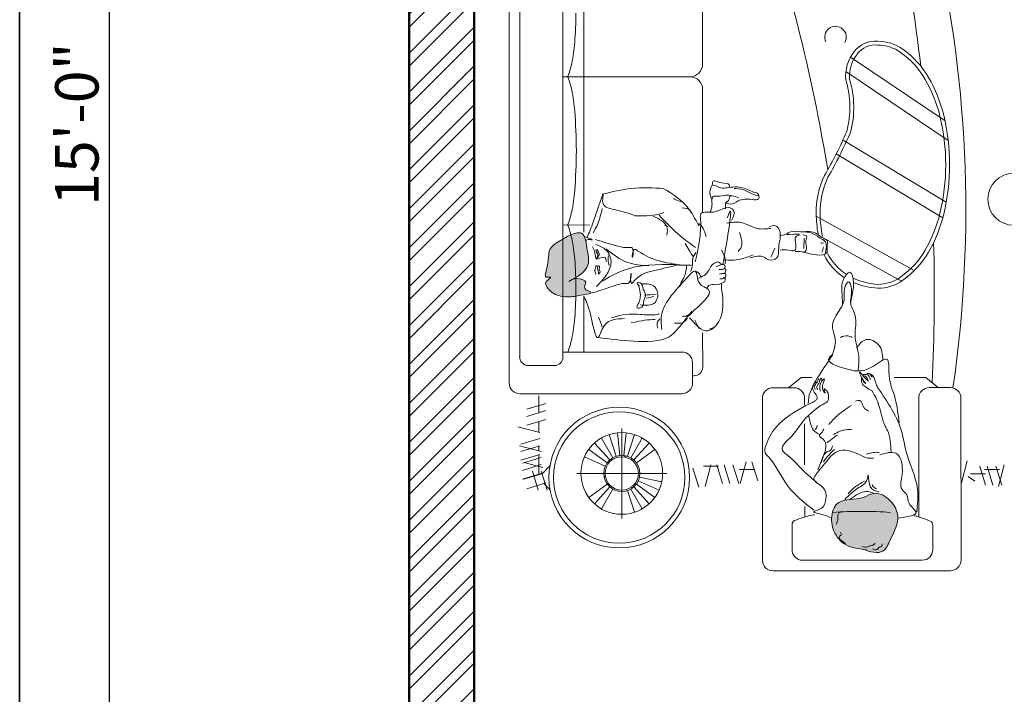
# Model space of a CAD drawing. Units: millimetres. Extents: x 20768 to 23556, y 50760 to 52704.
# Tile 16 of 36: x 21272 to 21408, y 51912 to 52005. Entities that reach past the tile are written whole.
import ezdxf

# ---------------------------------------------------------------- set-up
doc = ezdxf.new("R2010")
doc.units = ezdxf.units.MM
for name, color, linetype, lineweight in [('A-ANNO-TTLB', 7, 'Continuous', 35), ('A-FURN', 8, 'Continuous', 18), ('A-WALL', 7, 'Continuous', 50), ('A-WALL-PATT', 8, 'Continuous', 13), ('S-ANNO-DIMS', 2, 'Continuous', 18)]:
    doc.layers.add(name, color=color, linetype=linetype, lineweight=lineweight)
doc.styles.get("Standard").update_dxf_attribs({"font": 'arial.ttf'})
doc.dimstyles.new('ISO-25', dxfattribs={"dimtxt": 6, "dimasz": 2.5, "dimexe": 1.25, "dimexo": 0.625, "dimtad": 1, "dimdec": 0, "dimlunit": 3, "dimtxsty": 'Standard', "dimcen": 2.5, "dimadec": 0, "dimazin": 0, "dimtfac": 1, "dimtdec": 0, "dimtmove": 0, "dimatfit": 3, "dimfxl": 1, "dimarcsym": 0})

# ---------------------------------------------------------------- blocks, each defined once
blk = doc.blocks.new('A$C32DD204E')
at = {"ltscale": 3}
h = blk.add_hatch(color=256, dxfattribs=at)
edge = h.paths.add_edge_path()
edge.add_spline(control_points=[(248.5, 1171), (279.6, 1188.5), (331.5, 1220.4), (312.1, 1296.2), (303.9, 1374.7), (243.4, 1354.4), (209.2, 1331.9), (147.9, 1299.6), (163.4, 1244.6), (138.6, 1178), (180.2, 1188.1), (136, 1164), (157.4, 1133.7), (185.5, 1110.9), (241.5, 1099.6), (276.6, 1109.9), (350.3, 1120.6), (292.2, 1133.5), (320.4, 1170.6), (274.8, 1182.2), (255.2, 1174.5), (248.5, 1171)], knot_values=[6.92976, 6.92976, 6.92976, 6.92976, 88.633957, 150.80248, 204.81141, 248.139794, 279.389018, 321.893636, 408.375761, 431.643524, 447.144857, 469.07466, 497.305108, 522.125936, 570.063074, 628.708388, 656.922664, 684.873946, 704.64736, 740.083308, 760.727208, 760.727208, 760.727208, 760.727208], degree=3, periodic=0)
h = blk.add_hatch(color=256, dxfattribs=at)
edge = h.paths.add_edge_path()
edge.add_spline(control_points=[(1426.4, 86.6), (1397.7, 90.1), (1345.7, 99.1), (1298.9, 165.8), (1296.3, 225.7), (1328.2, 297.6), (1410.2, 279.3), (1477.3, 324.4), (1540.8, 288.1), (1580.5, 210.8), (1543, 141.8), (1506.8, 60.6), (1456.5, 76.7), (1426.4, 86.6)], knot_values=[11.171972, 11.171972, 11.171972, 11.171972, 83.935274, 146.390702, 207.043537, 236.474222, 338.687878, 374.142978, 438.985032, 497.846364, 587.349285, 634.808067, 704.959464, 704.959464, 704.959464, 704.959464], degree=3, periodic=0)
for p, q in [((0, 755.3, -685.7), (0.2, 2629.6, -685.7)), ((779.4, 2042.5, -685.7), (779.6, 2565.6, -685.7)), ((42.1, 861.2, -685.7), (42.7, 2524.3, -685.7)), ((216, 1393.9, -685.7), (216.2, 2524.2, -685.7)), ((301, 1394, -685.7), (301.2, 2504.1, -685.7)), ((1375.8, 2071.1, -685.7), (1756.4, 1813.8, -685.7)), ((216, 1991.7, -685.7), (595.7, 1991.5, -685.7)), ((595.7, 1991.5, -685.7), (728.3, 1991.5, -685.7)), ((1356.9, 2013.1, -685.7), (1769.1, 1734.5, -685.7)), ((779.4, 1940.4, -685.7), (779.4, 1445.2, -685.7)), ((1345.3, 1735.8, -685.7), (1761.4, 1485.6, -685.7)), ((1318.2, 1681.4, -685.7), (1747.5, 1423.2, -685.7)), ((1237.5, 1428.9, -685.7), (1632.1, 1210.6, -685.7)), ((216, 1394.2, -685.7), (216.2, 861.4, -685.7)), ((216, 1393.9, -685.7), (323, 1394, -685.7)), ((301, 1394.2, -685.7), (301, 1364.8, -685.7)), ((1245.7, 1353.6, -685.7), (1581.4, 1167.9, -685.7)), ((1188.7, 1340.5), (1187.5, 1298.8)), ((301.1, 1106.9, -685.7), (301.2, 881.5, -685.7)), ((370.5, 964.2), (368.9, 965.7)), ((779.5, 959.1, -685.7), (779.6, 820, -685.7)), ((216.2, 881.5, -685.7), (696.3, 881.7, -685.7)), ((738.8, 782.8, -685.7), (738.8, 839.2, -685.7)), ((76.8, 827.3, -685.7), (182.2, 827.3, -685.7)), ((739.1, 787, -685.7), (739.1, 756.3, -685.7)), ((739.1, 785.9, -685.7), (745.6, 785.9, -685.7)), ((1125.7, 738.2, -685.7), (1176, 779.7, -685.7)), ((1220.3, 779.7, -685.7), (1176, 779.7, -685.7)), ((1678.7, 779.9, -685.7), (1551.9, 779.9, -685.7)), ((1729.9, 737.7, -685.7), (1678.7, 779.9, -685.7)), ((1148, 738.2, -685.7), (1062.9, 738.1, -685.7)), ((1778.1, 738.4, -685.7), (1693.1, 738.4, -685.7)), ((42.8, 713.5, -685.7), (696.6, 713.7, -685.7)), ((147, 675, -685.7), (70.5, 651.5, -685.7)), ((1020.4, 695.6, -685.7), (1020.7, 42.5, -685.7)), ((1190.5, 669.7, -685.7), (1190.5, 695.7, -685.7)), ((1650.7, 217.2, -685.7), (1650.6, 695.8, -685.7)), ((1820.9, 42.8, -685.7), (1820.7, 695.9, -685.7)), ((147, 645.6, -685.7), (70.5, 622.1, -685.7)), ((147, 610.3, -685.7), (70.5, 586.8, -685.7)), ((123.5, 557.3, -685.7), (35.3, 580.9, -685.7)), ((446, 465, -685.7), (436.4, 556.4, -685.7)), ((453.6, 392.6, -685.7), (453.6, 574.3, -685.7)), ((461.2, 465, -685.7), (470.8, 556.4, -685.7)), ((1190.6, 427.1, -685.7), (1190.6, 592.2, -685.7)), ((123.5, 533.8, -685.7), (47, 510.3, -685.7)), ((417.2, 455.6, -685.7), (371.3, 535.2, -685.7)), ((431.1, 461.8, -685.7), (402.7, 549.2, -685.7)), ((476.1, 461.8, -685.7), (504.5, 549.2, -685.7)), ((490, 455.6, -685.7), (536, 535.2, -685.7)), ((129.3, 480.9, -685.7), (41.1, 504.4, -685.7)), ((123.5, 504.4, -685.7), (47, 480.9, -685.7)), ((394.8, 435.4, -685.7), (320.4, 489.4, -685.7)), ((404.9, 446.7, -685.7), (343.4, 515, -685.7)), ((502.3, 446.7, -685.7), (563.8, 515, -685.7)), ((512.5, 435.4, -685.7), (586.9, 489.4, -685.7)), ((123.5, 469.1, -685.7), (47, 445.6, -685.7)), ((129.3, 457.3, -685.7), (52.9, 433.8, -685.7)), ((387.1, 422.2, -685.7), (303.2, 459.6, -685.7)), ((469.9, 463.5, -685.7), (465.2, 458.8, -685.7)), ((954.3, 439.6, -685.7), (930.7, 351.4, -685.7)), ((977.8, 439.6, -685.7), (1001.3, 363.1, -685.7)), ((1822.4, 354.9, -685.7), (1846, 443.1, -685.7)), ((129.3, 427.9, -685.7), (52.9, 404.4, -685.7)), ((135.2, 416.2, -685.7), (60.4, 436.1, -685.7)), ((117, 325.5, -685.7), (93.5, 401.9, -685.7)), ((152.3, 325.5, -685.7), (128.8, 401.9, -685.7)), ((163.9, 422.7, -685.7), (132.1, 390.9, -685.7)), ((764.1, 337.3, -685.7), (740.6, 413.7, -685.7)), ((783.1, 421.6), (843.8, 421.6)), ((813.1, 427.8, -685.7), (789.5, 339.6, -685.7)), ((836.6, 427.8, -685.7), (860.1, 351.4, -685.7)), ((866, 427.8, -685.7), (889.5, 351.4, -685.7)), ((901.3, 427.8, -685.7), (924.8, 351.4, -685.7)), ((928.1, 408.1), (988.8, 408.1)), ((1896.4, 421.9, -685.7), (1920, 345.5, -685.7)), ((1915.9, 408.1), (1976.6, 408.1)), ((1925.8, 421.9, -685.7), (1949.4, 345.5, -685.7)), ((1961.1, 421.9, -685.7), (1984.7, 345.5, -685.7)), ((1995.1, 427.8, -685.7), (1971.6, 339.6, -685.7)), ((129.3, 392.6, -685.7), (52.9, 369.1, -685.7)), ((135.2, 392.6, -685.7), (58.8, 369.1, -685.7)), ((453.6, 392.6, -685.7), (271.9, 392.6, -685.7)), ((387.4, 381, -685.7), (382.7, 376.3, -685.7)), ((453.6, 392.6, -685.7), (453.6, 210.9, -685.7)), ((453.6, 392.6, -685.7), (635.4, 392.6, -685.7)), ((520.1, 363, -685.7), (604.1, 325.6, -685.7)), ((524.8, 377.5, -685.7), (614.7, 358.3, -685.7)), ((1849.9, 380.2, -685.7), (1876.3, 360.8, -685.7)), ((1858.6, 391.3), (1919.3, 391.3)), ((147, 354.5, -685.7), (70.5, 331, -685.7)), ((139.9, 352.3, -685.7), (164.1, 328, -685.7)), ((394.8, 349.8, -685.7), (320.4, 295.8, -685.7)), ((404.9, 338.5, -685.7), (343.4, 270.2, -685.7)), ((417.2, 329.6, -685.7), (371.3, 249.9, -685.7)), ((476.1, 323.4, -685.7), (504.5, 235.9, -685.7)), ((490, 329.6, -685.7), (536, 249.9, -685.7)), ((502.3, 338.5, -685.7), (563.8, 270.2, -685.7)), ((512.5, 349.8, -685.7), (586.9, 295.8, -685.7)), ((1190.7, 217.1, -685.7), (1190.7, 258.6, -685.7)), ((1139.7, 85.1, -685.7), (1139.7, 186.8, -685.7)), ((1707.1, 85.3, -685.7), (1707, 184.5, -685.7)), ((1182.2, 42.6, -685.7), (1664.6, 42.8, -685.7)), ((1063.2, 0, -685.7), (1778.4, 0.3, -685.7))]:
    blk.add_line(p, q)
at = {"elevation": -685.7}
for points in [[(234.8, 1392.4, 0.047423), (251.7, 1447.7, 0.029233), (263.9, 1532.1, 0.017749), (270.5, 1692.8, 0.02107)], [(234.8, 1395.5, -0.047423), (251.7, 1340.2, -0.029233), (263.9, 1255.7, -0.02107), (268.9, 1137.6, -0.02107)], [(236, 1394.2, -0.00246), (234.8, 1391.4)], [(268.9, 1137.6, -0.02107), (264, 1019.4, -0.029233), (251.9, 935, -0.045778), (235.8, 881.5, -0.201615)]]:
    blk.add_lwpolyline(points, format="xyb", dxfattribs=at)
for points in [[(119.4, 705.9), (119.4, 637.1)], [(119.4, 601.8), (119.4, 558.4)], [(119.4, 503.2), (119.4, 483.5)], [(119.4, 467.9), (119.4, 387.8)]]:
    blk.add_lwpolyline(points, dxfattribs=at)
for centre, radius in [((2033.7, 1497.8, -685.7), 104.7), ((443.5, 376, -685.7), 283.5), ((443.5, 376, -685.7), 264.6), ((453.6, 392.6, -685.7), 164.7), ((453.6, 392.6, -685.7), 72.8), ((453.6, 392.6, -685.7), 67.2)]:
    blk.add_circle(centre, radius)
for centre, radius, start, end in [((-3160.4, 1453.5, -685.7), 5000.5, 351.7639, 13.5399), ((-5717.4, 460.8, -685.7), 7095.9, 9.37507, 17.5955), ((-6034.3, 1118.6, -685.7), 7747.5, 6.78419, 11.06631), ((-1135.1, 2248.6, -685.7), 1404, 355.1489, 359.9772), ((1315, 2151.6, -685.7), 43.3, 329.4196, 206.4089), ((-463.5, 2191.6, -685.7), 730, 348.451, 355.1489), ((1474.3, 2030.8, -685.7), 104.3, 83.9251, 143.2199), ((1474.3, 2030.8, -685.7), 88.8, 83.3999, 143.3893), ((1485.3, 1960, -685.7), 159, 54.5394, 90.3034), ((1485.3, 1960, -685.7), 174.6, 54.5394, 90), ((1514.9, 1993.6, -685.7), 159.2, 141.263, 185.4473), ((1514.9, 1993.6, -685.7), 143.6, 141.1552, 184.8436), ((1375.6, 1805.9, -685.7), 348.1, 30.1802, 54.5394), ((1375.6, 1805.9, -685.7), 363.7, 30.1802, 54.5394), ((-47.7, 2106.6, -685.7), 305.7, 337.5906, 348.451), ((728.3, 2042.5, -685.7), 51, 269.9772, 359.9772), ((-47.8, 1877.9, -685.7), 305.7, 21.7999, 22.3637), ((-47.7, 1876.7, -685.7), 305.7, 11.549, 22.4094), ((728.3, 1940.4, -685.7), 51, 0.0228, 90.0228), ((1200.1, 1703.8, -685.7), 566.7, 13.5438, 30.1802), ((993.4, 1867.9, -685.7), 379.5, 345.261, 16.9432), ((993.4, 1867.9, -685.7), 395.1, 345.0883, 16.7074), ((1200.1, 1703.8, -685.7), 551.1, 13.5438, 30.1802), ((-463.5, 1791.7, -685.7), 730, 4.8511, 11.549), ((-1995, 1680, -685.7), 2265.5, 0.3248, 4.3921), ((921.7, 1636.8, -685.7), 837.4, 0, 13.5438), ((921.7, 1636.8, -685.7), 853, 0, 13.5438), ((-174.4, 2435.8, -685.7), 1672.4, 329.7762, 336.5922), ((-174.4, 2435.8, -685.7), 1688, 329.7992, 336.632), ((921.7, 1636.8, -685.7), 837.4, 346.4562, 0), ((921.7, 1636.8, -685.7), 853, 346.4562, 0), ((1584.9, 1445.2, -685.7), 347.6, 154.6827, 181.0708), ((1584.9, 1445.2, -685.7), 332, 154.7964, 181.089), ((1699.8, 1441.1, -685.7), 462.4, 180.2965, 190.3289), ((1699.8, 1441.1, -685.7), 446.9, 180.283, 192.0106), ((1200.1, 1569.7, -685.7), 551.1, 329.8198, 346.4562), ((1200.1, 1569.7, -685.7), 566.7, 329.8198, 346.4562), ((464.9, -539.7), 1961.2, 81.0036, 81.3607), ((631.8, -596.5), 1995.1, 85.9802, 86.2563), ((-6034.3, 1118.6, -685.7), 7747.5, 357.33463, 1.51542), ((1486, 1384.5, -685.7), 244, 207.1509, 235.8302), ((1486, 1384.5, -685.7), 228.4, 207.3492, 235.7987), ((1375.6, 1467.7, -685.7), 348.1, 305.4606, 329.8198), ((1375.6, 1467.7, -685.7), 363.7, 305.4606, 329.8198), ((1509.1, 1466.2, -685.7), 312.4, 247.051, 265.7344), ((1509.1, 1466.2, -685.7), 328, 248.6473, 265.8394), ((1485.3, 1313.6, -685.7), 174.6, 270, 305.4606), ((1485.3, 1313.6, -685.7), 159, 270.2019, 305.4606), ((696.3, 839.1, -685.7), 42.5, 0.0228, 90.0228), ((77.2, 862.5, -685.7), 35.2, 177.8872, 269.238), ((182.2, 861.4, -685.7), 34, 270.0228, 0.0228), ((745.5, 820, -685.7), 34, 270.0228, 0.0228), ((42.9, 756.4, -685.7), 42.9, 178.4457, 269.7882), ((696.5, 756.3, -685.7), 42.5, 270.0228, 0.0228), ((1063, 695.6, -685.7), 42.5, 90.0228, 180.0228), ((1148, 695.6, -685.7), 42.5, 0.0228, 90.0228), ((1693.1, 695.9, -685.7), 42.5, 90.0228, 180.0228), ((1778.1, 695.9, -685.7), 42.5, 0.0228, 90.0228), ((1421.2, -1279.2, -685.7), 1518.9, 90.0228, 94.419), ((1421.2, -1279.2, -685.7), 1518.9, 85.6266, 90.0228), ((1156.7, 186.8, -685.7), 17, 113.7374, 180.0228), ((1280.5, -94.8, -685.7), 324.6, 100.5374, 113.7374), ((1364.6, -547, -685.7), 784.5, 99.8363, 100.5374), ((1560.9, -94.7, -685.7), 324.6, 65.1817, 77.2735), ((1690, 184.5, -685.7), 17, 0.0228, 65.1817), ((1182.2, 85.1, -685.7), 42.5, 180.0228, 270.0228), ((1664.6, 85.3, -685.7), 42.5, 270.0228, 0.0228), ((1063.2, 42.5, -685.7), 42.5, 180.0228, 270.0228), ((1778.4, 42.8, -685.7), 42.5, 270.0228, 0.0228)]:
    blk.add_arc(centre, radius, start, end)
at = {"ltscale": 3}
for centre, radius, start, end in [((1357, 906.6), 40.6, 79.5148, 123.0894), ((1352, 880), 67.7, 63.6392, 79.5148)]:
    blk.add_arc(centre, radius, start, end, dxfattribs=at)
for points, knots in [([(815.6, 1499.7), (813.2, 1505.1), (807.5, 1517.9), (809.7, 1535.9), (818.3, 1563.8), (849.5, 1539.3), (888.8, 1546.3), (939.9, 1551.3), (976, 1527), (1006.1, 1522.5), (1011, 1491), (964.4, 1500), (925.8, 1499.2), (898.4, 1471.9), (869.3, 1485.1), (891, 1492.1), (886, 1512.2), (894.6, 1511.6), (895.6, 1511.5)], [0, 0, 0, 0, 15.214729, 36.055512, 48.857472, 79.738512, 103.122769, 157.685733, 206.194273, 214.411126, 234.296897, 257.825245, 307.464974, 341.56748, 352.042995, 362.192251, 380.803332, 383.401633, 383.401633, 383.401633, 383.401633]), ([(817.1, 1553), (818.2, 1556.2), (819.7, 1561), (820, 1579.5), (854.5, 1556.5), (888.8, 1565.3), (887.1, 1549.5), (886.7, 1545.6)], [0, 0, 0, 0, 9.109215, 13.285838, 44.707752, 72.752889, 81.852859, 81.852859, 81.852859, 81.852859]), ([(314.5, 1345.5), (321.9, 1362.7), (341.1, 1407.4), (387.3, 1556.5), (369.3, 1464.2), (445.2, 1454.4), (487.7, 1439.1), (511.9, 1430.4)], [0, 0, 0, 0, 60.518576, 156.742964, 182.299185, 237.275016, 309.902587, 309.902587, 309.902587, 309.902587]), ([(374.5, 1517.7), (413.9, 1527.5), (495.5, 1547.9), (579.6, 1543.7), (622.9, 1541.5)], [0, 0, 0, 0, 106.409885, 220.025525, 220.025525, 220.025525, 220.025525]), ([(623, 1540.2), (656.5, 1519.3), (716.8, 1481.5), (749.4, 1418.6), (764, 1390.6)], [0, 0, 0, 0, 101.553402, 183.196527, 183.196527, 183.196527, 183.196527]), ([(809.7, 1446.3), (813.1, 1455.2), (819.4, 1471.8), (815.4, 1492.1), (820.4, 1513), (846.6, 1507.3), (878.7, 1519.8), (907.7, 1510), (925.2, 1504.1)], [0, 0, 0, 0, 24.284632, 45.084884, 56.190964, 71.83444, 101.967681, 148.338712, 148.338712, 148.338712, 148.338712]), ([(906, 1541.1), (918.1, 1540.7), (943.5, 1539.6), (973.1, 1520.3), (994.7, 1514.1), (1003.7, 1511.5)], [0, 0, 0, 0, 31.421868, 65.723795, 90.374568, 90.374568, 90.374568, 90.374568]), ([(662.7, 1500.2), (666.7, 1498), (679.3, 1491.4), (693.1, 1487.5), (702.4, 1484.9)], [0, 0, 0, 0, 12.001288, 37.458402, 37.458402, 37.458402, 37.458402]), ([(895.2, 1411.9), (903.3, 1427.4), (912.7, 1445.6), (880, 1477.1), (837.9, 1433.9), (767.6, 1451.2), (776.7, 1361.9), (762.8, 1301.5), (749.8, 1245.2)], [0, 0, 0, 0, 37.77004, 44.330448, 112.206702, 158.127425, 169.373671, 326.046663, 326.046663, 326.046663, 326.046663]), ([(861.3, 1235.3), (864.2, 1253), (878.2, 1331.2), (903.8, 1491.5), (882.2, 1430.6), (879.3, 1422.5)], [229.252261, 229.252261, 229.252261, 229.252261, 259.312026, 344.867622, 358.082672, 358.082672, 358.082672, 358.082672]), ([(871.9, 1484.8), (871.9, 1477.9), (871.9, 1469.5), (871.9, 1461.1), (871.9, 1459.6)], [0, 0, 0, 0, 18.199941, 22.100035, 22.100035, 22.100035, 22.100035]), ([(338.4, 1362.4), (345, 1374.5), (361.7, 1405.4), (370, 1439.6), (375.1, 1460.4)], [0, 0, 0, 0, 36.019014, 92.081432, 92.081432, 92.081432, 92.081432]), ([(505.6, 1431.2), (538.2, 1430.5), (578.2, 1429.6), (616, 1441.7), (623, 1444)], [0, 0, 0, 0, 84.476355, 104.032988, 104.032988, 104.032988, 104.032988]), ([(580.1, 1429.8), (591.5, 1424.4), (612.6, 1414.6), (640.6, 1388.2), (637, 1365), (635.1, 1353.2)], [0, 0, 0, 0, 33.626167, 62.160116, 91.695701, 91.695701, 91.695701, 91.695701]), ([(603.8, 1433.3), (631.3, 1404.4), (676.7, 1356.7), (730.1, 1318.2), (751.2, 1303)], [0, 0, 0, 0, 104.676597, 172.875133, 172.875133, 172.875133, 172.875133]), ([(696.3, 1463.4), (710.4, 1462.2), (728.4, 1460.6), (732.2, 1445.3), (733, 1442)], [0, 0, 0, 0, 31.408902, 39.899476, 39.899476, 39.899476, 39.899476]), ([(772.8, 1393), (778.4, 1384.1), (787.5, 1369.7), (792.4, 1353.3), (794.2, 1347.1)], [0, 0, 0, 0, 27.640179, 44.620551, 44.620551, 44.620551, 44.620551]), ([(877.4, 1401.3), (897.1, 1404.5), (939.9, 1411.6), (993.7, 1373.5), (1035.6, 1378.1), (1054.5, 1380.1)], [0, 0, 0, 0, 51.063738, 110.501338, 159.193788, 159.193788, 159.193788, 159.193788]), ([(969.9, 1261.1), (990.7, 1266.8), (1019.1, 1274.6), (1048.1, 1247.4), (1089.5, 1258.3), (1081.3, 1314.7), (1101.6, 1357.4), (1073.7, 1397.1), (1055.9, 1389.4), (1046.5, 1385.4)], [0, 0, 0, 0, 51.063966, 69.760857, 98.442485, 136.21289, 196.583877, 217.96974, 241.616381, 241.616381, 241.616381, 241.616381]), ([(240.5, 1166.5), (274.5, 1185.5), (332.2, 1217.8), (312.1, 1296.2), (303.9, 1374.7), (243.4, 1354.4), (209.2, 1331.9), (147.9, 1299.6), (163.4, 1244.6), (138.6, 1178), (180.2, 1188.1), (136, 1164), (157.4, 1133.7), (185.5, 1110.9), (241.5, 1099.6), (276.6, 1109.9), (350.3, 1120.6), (292.2, 1133.5), (320.4, 1170.6), (269.8, 1183.5), (249.6, 1171.8), (240.5, 1166.5)], [0, 0, 0, 0, 88.633957, 150.80248, 204.81141, 248.139794, 279.389018, 321.893636, 408.375761, 431.643524, 447.144857, 469.07466, 497.305108, 522.125936, 570.063074, 628.708388, 656.922664, 684.873946, 704.64736, 740.083308, 769.084366, 769.084366, 769.084366, 769.084366]), ([(927.6, 1364.2), (935.3, 1341.3), (945, 1312.2), (926.2, 1291.8), (922.3, 1287.5)], [0, 0, 0, 0, 55.878701, 70.732003, 70.732003, 70.732003, 70.732003]), ([(1094.1, 1351), (1103.8, 1352.9), (1123.3, 1356.8), (1183.4, 1359.1), (1146, 1345.7), (1156.4, 1319.3), (1156, 1283.3), (1121, 1296.3), (1102.2, 1294.1), (1091.5, 1292.8)], [0, 0, 0, 0, 32.791493, 65.856029, 77.112898, 107.365096, 127.973901, 150.397914, 180.540849, 180.540849, 180.540849, 180.540849]), ([(1118, 1358.2), (1121.8, 1360.9), (1138, 1372), (1178.1, 1363), (1230.2, 1373), (1257, 1342.7), (1288.6, 1331.3), (1278.1, 1306), (1286.4, 1273), (1223.1, 1270.5), (1188.8, 1286.7), (1158.9, 1287.5), (1151.8, 1287.7)], [0, 0, 0, 0, 12.05449, 50.662285, 100.751119, 139.349436, 152.871984, 178.39508, 194.636814, 232.879132, 291.995735, 310.219291, 310.219291, 310.219291, 310.219291]), ([(1183.4, 1354.2), (1190.9, 1352.9), (1203.6, 1350.5), (1189.2, 1323.8), (1204.2, 1303.5), (1191.8, 1283.5), (1185.8, 1284.4), (1183.1, 1284.9)], [0, 0, 0, 0, 15.405528, 26.125312, 63.82535, 72.147315, 78.642841, 78.642841, 78.642841, 78.642841]), ([(1190.6, 1366.4), (1202.4, 1365), (1228.5, 1361.8), (1250.9, 1340.1), (1273.6, 1330.7), (1281.3, 1309.2), (1276.7, 1293.2), (1273.5, 1281.9)], [0, 0, 0, 0, 30.578618, 67.353333, 79.611572, 92.413964, 122.566762, 122.566762, 122.566762, 122.566762]), ([(309.6, 1329.3), (310.5, 1331), (315, 1339.5), (351.8, 1328.4), (322, 1340.1), (304, 1347.2)], [0, 0, 0, 0, 4.957486, 24.33421, 53.851131, 53.851131, 53.851131, 53.851131]), ([(348, 1335.2), (378.1, 1325.8), (423.4, 1311.5), (470.9, 1300.8), (505.7, 1306.7), (492.8, 1231.6), (496.4, 1304.6), (545.6, 1270.4), (599.6, 1246.5), (663.3, 1236.7), (694.3, 1232)], [0, 0, 0, 0, 82.179012, 124.172551, 131.128421, 166.009294, 194.708047, 207.195703, 291.828264, 372.00922, 372.00922, 372.00922, 372.00922]), ([(348.4, 1315.8), (363.7, 1309.9), (395.9, 1297.5), (418.6, 1242), (392.1, 1188.2), (365.5, 1160.4), (351.7, 1146)], [0, 0, 0, 0, 41.941762, 88.289003, 137.229401, 190.028503, 190.028503, 190.028503, 190.028503]), ([(335.3, 1306), (339.3, 1299.3), (347.7, 1285.3), (345.8, 1247.6), (369.4, 1263.9), (388.2, 1265.3), (389.8, 1254.3), (390.8, 1247.2)], [0, 0, 0, 0, 21.811235, 45.429417, 66.268319, 74.855405, 90.278481, 90.278481, 90.278481, 90.278481]), ([(350.6, 1295.1), (350.5, 1293), (349.7, 1284.3), (361.3, 1275.9), (349.4, 1255.1), (369.1, 1276.1), (357.7, 1286), (354.6, 1293), (353.7, 1295.1)], [0, 0, 0, 0, 5.37014, 22.350864, 30.841366, 44.263375, 58.721741, 64.724876, 64.724876, 64.724876, 64.724876]), ([(390.3, 1298.1), (418.1, 1276), (468.7, 1235.6), (533, 1231.3), (562.2, 1229.4)], [0, 0, 0, 0, 90.713488, 165.812862, 165.812862, 165.812862, 165.812862]), ([(399.6, 1270.6), (398.4, 1260.2), (396.8, 1246.5), (401.5, 1233.8), (402.6, 1230.8)], [0, 0, 0, 0, 26.8507, 35.340922, 35.340922, 35.340922, 35.340922]), ([(751.4, 1282.8), (746.1, 1274), (734.5, 1254.2), (741, 1225.1), (732.3, 1210.3), (730, 1206.3)], [0, 0, 0, 0, 26.441749, 58.774114, 70.780485, 70.780485, 70.780485, 70.780485]), ([(855.4, 1292), (862.2, 1280.1), (872.2, 1262.7), (871, 1243.1), (870.7, 1236.9)], [0, 0, 0, 0, 34.902027, 51.012448, 51.012448, 51.012448, 51.012448]), ([(864.1, 1253.2), (886.5, 1252.3), (927.8, 1250.7), (965.7, 1266.9), (983.1, 1274.3)], [0, 0, 0, 0, 58.013512, 107.149157, 107.149157, 107.149157, 107.149157]), ([(334.8, 1120.9), (360.4, 1128.3), (405.8, 1141.5), (452.6, 1160.2), (491.3, 1155.9), (493, 1241.6), (484.9, 1142.7), (524.3, 1197.5), (588.2, 1210.9), (652.5, 1226.4), (686.4, 1234.7)], [0, 0, 0, 0, 70.409867, 124.986685, 129.624235, 168.516696, 205.713361, 218.8346, 299.734666, 390.28545, 390.28545, 390.28545, 390.28545]), ([(351.7, 1230.9), (348.5, 1224.4), (342.8, 1212.8), (346.7, 1200.5), (348.4, 1195)], [0, 0, 0, 0, 18.113831, 32.718438, 32.718438, 32.718438, 32.718438]), ([(356.8, 1230.8), (356.3, 1225.5), (355.3, 1214.9), (360.7, 1205.6), (359.1, 1194), (370.8, 1206.3), (359, 1213.3), (366.7, 1228.5), (361, 1227.9), (359.8, 1227.7)], [0, 0, 0, 0, 13.425536, 27.116244, 29.801129, 37.393081, 48.463136, 59.203416, 61.886553, 61.886553, 61.886553, 61.886553]), ([(371.8, 1165.9), (400.4, 1182.7), (490.8, 1235.8), (597.5, 1235.1), (670.5, 1234.7)], [0, 0, 0, 0, 86.085059, 272.751702, 272.751702, 272.751702, 272.751702]), ([(760.7, 1178.5), (777.8, 1186), (795.8, 1193.8), (808.8, 1220.7), (817.6, 1235.9), (839.6, 1248.1), (848.9, 1241.2), (853.6, 1237.7)], [0, 0, 0, 0, 45.537019, 47.905206, 78.191519, 91.952902, 106.155728, 106.155728, 106.155728, 106.155728]), ([(796.9, 1139.9), (800.1, 1144.8), (807.4, 1155.9), (834.8, 1150.8), (858.6, 1157), (872.2, 1171.5), (868.5, 1186.6), (860.5, 1174.8), (843.8, 1177.9), (862.3, 1176.4), (874.3, 1181.8), (871.9, 1204.3), (860, 1196.4), (840.8, 1196.3), (860.8, 1197.9), (873.3, 1198.7), (874, 1221), (859.5, 1214.2), (834.1, 1215.5), (865.4, 1212.3), (872.4, 1225.4), (866.1, 1236.7), (854.1, 1234.8), (844.5, 1230), (838, 1227.2), (834.3, 1225.6)], [0, 0, 0, 0, 14.245589, 32.27085, 65.424938, 75.415665, 83.125969, 92.594533, 101.062211, 108.471373, 123.178778, 136.06387, 144.792436, 155.430033, 166.067631, 176.109786, 189.879186, 198.412834, 212.213818, 230.332194, 238.870274, 247.408355, 257.993066, 266.055047, 276.480967, 276.480967, 276.480967, 276.480967]), ([(359.2, 940.8), (405, 934.5), (496.9, 921.8), (657.2, 922.9), (708.4, 1030.4), (845.8, 1129.3), (754.4, 1150.7), (759.2, 1230.2), (662.8, 1120.6), (605, 1063.1), (613.7, 984.5), (615, 972.8)], [0, 0, 0, 0, 125.422801, 251.68088, 363.259103, 469.510953, 507.917449, 552.801864, 594.966396, 768.088902, 798.341471, 798.341471, 798.341471, 798.341471]), ([(714.7, 1227.7), (712.6, 1210.6), (709.9, 1187.3), (691.9, 1163.5), (688.8, 1151.4), (687.1, 1145.1)], [0, 0, 0, 0, 44.281186, 59.934993, 76.915365, 76.915365, 76.915365, 76.915365]), ([(749.9, 1207.5), (755.3, 1205.7), (765.7, 1202.1), (769.7, 1191.9), (771.6, 1186.9)], [0, 0, 0, 0, 14.202992, 27.472435, 27.472435, 27.472435, 27.472435]), ([(1343.7, 1073.5), (1342.6, 1091.5), (1340.7, 1125.6), (1338.5, 1168.8), (1378.1, 1222.7), (1390.8, 1161.5), (1384.6, 1125), (1379.2, 1097.9), (1376.2, 1082.4)], [0, 0, 0, 0, 46.697433, 88.465151, 123.324676, 161.835136, 191.877979, 232.626852, 232.626852, 232.626852, 232.626852]), ([(518.9, 1154.3), (526.9, 1132.1), (537.4, 1103.2), (507.2, 1054.7), (545.6, 1061.6), (538.1, 1089.1), (555, 1112.1), (536.7, 1133.8), (538, 1161.8), (509.4, 1162.3), (519.4, 1153.2), (525, 1148.2)], [0, 0, 0, 0, 64.497154, 84.043581, 100.365205, 128.396624, 142.854646, 168.325592, 192.338234, 203.071238, 216.493247, 216.493247, 216.493247, 216.493247]), ([(534.2, 1157.3), (554.1, 1157.1), (589.5, 1156.6), (603.8, 1109.4), (582.9, 1067.4), (550.3, 1069.9), (528.1, 1071.6)], [0, 0, 0, 0, 46.862522, 83.38104, 107.393682, 159.00759, 159.00759, 159.00759, 159.00759]), ([(726.7, 1020.4), (751.1, 991.9), (795, 940.9), (875.3, 1034.1), (857.4, 1111.5), (854.9, 1152.3), (854.7, 1157.9)], [0, 0, 0, 0, 53.201817, 95.441996, 166.7115, 178.37996, 178.37996, 178.37996, 178.37996]), ([(1299.3, 863.8), (1308, 886.5), (1318.6, 914), (1309.4, 955.4), (1287.5, 1011.9), (1362.9, 1071.8), (1344.1, 1129.9), (1369.3, 1179.2), (1386.1, 1119.1), (1366.1, 1080.1), (1406.2, 1020.5), (1384.3, 946.3), (1413.8, 873.4), (1408.1, 824.6), (1405.7, 804.8)], [0, 0, 0, 0, 60.970115, 74.178445, 111.267097, 210.963126, 255.074467, 279.515708, 307.41666, 359.287359, 403.554034, 473.492101, 549.720465, 601.59141, 601.59141, 601.59141, 601.59141]), ([(300.5, 1107.7), (308.7, 1090.3), (330.5, 1043.9), (351.6, 894), (382, 1013), (432.6, 1015.3), (464.2, 1016.7)], [0, 0, 0, 0, 58.099529, 155.224826, 201.006913, 277.065022, 277.065022, 277.065022, 277.065022]), ([(411.8, 1019.6), (427, 1024.3), (457.8, 1033.9), (515.9, 1036.8), (565, 1028.3), (597.4, 1033.7), (604.5, 1034.9)], [0, 0, 0, 0, 41.657024, 84.672483, 151.807143, 170.780764, 170.780764, 170.780764, 170.780764]), ([(696.3, 1025.7), (703.9, 1025.8), (720.6, 1026), (730.6, 1039.7), (736.1, 1047.2)], [0, 0, 0, 0, 18.973621, 41.74948, 41.74948, 41.74948, 41.74948]), ([(490.8, 999.2), (519.7, 1005.6), (552.1, 1012.8), (585.1, 1012.5), (588.6, 1012.5)], [0, 0, 0, 0, 77.391086, 86.66573, 86.66573, 86.66573, 86.66573]), ([(607.1, 1015.1), (602.5, 1010.1), (592.9, 999.4), (597, 985.4), (599.2, 978.1)], [0, 0, 0, 0, 16.728024, 35.434645, 35.434645, 35.434645, 35.434645]), ([(665.7, 998.2), (677.7, 997.4), (698.1, 996), (712, 1010.5), (717.7, 1016.5)], [0, 0, 0, 0, 29.637545, 50.599936, 50.599936, 50.599936, 50.599936]), ([(806.4, 973.7), (817.2, 977.3), (832.6, 982.5), (838.3, 996.9), (840.1, 1001.2)], [0, 0, 0, 0, 27.630169, 39.636541, 39.636541, 39.636541, 39.636541]), ([(1506.2, 849.1), (1504.6, 871.7), (1501.6, 913.4), (1435.1, 944.4), (1411.3, 913.9), (1399.8, 899.3)], [0, 0, 0, 0, 56.575903, 104.225618, 148.354052, 148.354052, 148.354052, 148.354052]), ([(1204.8, 674.8), (1205.7, 689.1), (1209.7, 751.6), (1334.2, 902.6), (1270.1, 841.7), (1388.3, 800.1), (1443.9, 802.3), (1533.8, 875.3), (1524.6, 770.6), (1559.6, 702.9), (1567.5, 630.9), (1571.2, 598.1)], [0, 0, 0, 0, 42.167956, 184.846032, 188.510605, 261.118314, 357.582537, 412.070511, 453.838275, 554.467695, 638.871943, 638.871943, 638.871943, 638.871943]), ([(1436.7, 754.6), (1431.6, 760.9), (1422.6, 772.2), (1405.8, 809.4), (1424.2, 788.6), (1433.1, 777), (1442.7, 769.2), (1448, 764.8)], [0, 0, 0, 0, 25.892768, 46.183307, 59.392839, 73.451861, 90.844376, 90.844376, 90.844376, 90.844376]), ([(1463.3, 780.1), (1459.8, 786.6), (1454.5, 796.5), (1444.2, 795.2), (1440.6, 794.8)], [0, 0, 0, 0, 16.968689, 25.728505, 25.728505, 25.728505, 25.728505]), ([(1484.6, 738.9), (1481.6, 745.2), (1474.5, 760.5), (1471.1, 786), (1456, 792.4), (1450.6, 794.8)], [0, 0, 0, 0, 18.740722, 44.970985, 59.745283, 59.745283, 59.745283, 59.745283]), ([(1218.4, 676.9), (1223.2, 679.4), (1231.2, 683.6), (1246.3, 695.5), (1231.8, 715.6), (1217.1, 738.3), (1228.1, 756.3), (1234.4, 766.5)], [0, 0, 0, 0, 14.897426, 24.638003, 44.249327, 65.81281, 94.158391, 94.158391, 94.158391, 94.158391]), ([(1234.4, 766.5), (1235.6, 760.9), (1237.7, 752), (1226.1, 742.5), (1230.5, 735.3), (1233.1, 731.2)], [0, 0, 0, 0, 13.770952, 22.047872, 32.93541, 32.93541, 32.93541, 32.93541]), ([(1242.2, 729.9), (1240.7, 735.4), (1237.1, 749.3), (1256.2, 758.7), (1246.7, 779), (1243.7, 762.6), (1238.7, 758), (1235.9, 755.4)], [0, 0, 0, 0, 13.81853, 34.349896, 42.048978, 50.626809, 61.603847, 61.603847, 61.603847, 61.603847]), ([(1286.8, 709.7), (1285.8, 714.2), (1283.9, 723.2), (1262.2, 742.3), (1280.9, 705.6), (1248.4, 742.3), (1280.4, 780.7), (1262.2, 768.8), (1255.4, 758.3), (1249.3, 741.3), (1253, 729.3), (1254.6, 724)], [0, 0, 0, 0, 13.622009, 27.045047, 42.301032, 59.74223, 94.71225, 98.491569, 110.440566, 128.701216, 142.844466, 142.844466, 142.844466, 142.844466]), ([(1253.4, 768.2), (1254.3, 772.5), (1256.4, 781.6), (1262.5, 768.1), (1259.2, 764.5), (1258.1, 763.5)], [0, 0, 0, 0, 7.980072, 16.932683, 20.710806, 20.710806, 20.710806, 20.710806]), ([(1460.8, 726.5), (1456.3, 728), (1446.4, 731.4), (1435.3, 745.4), (1416.8, 751.9), (1420.5, 787.5), (1425.8, 764.3), (1431.5, 757.8), (1435, 755.6), (1436.7, 754.6)], [0, 0, 0, 0, 12.228513, 27.193094, 45.006155, 62.152179, 75.922416, 81.425571, 86.507745, 86.507745, 86.507745, 86.507745]), ([(1454.6, 771.5), (1452.3, 779.3), (1448, 793.7), (1433.4, 792), (1426.6, 791.2)], [0, 0, 0, 0, 18.54008, 34.34859, 34.34859, 34.34859, 34.34859]), ([(1446, 765.9), (1444.7, 770.8), (1442.8, 778), (1437.4, 782.8), (1435.6, 784.3)], [0, 0, 0, 0, 12.899473, 18.839157, 18.839157, 18.839157, 18.839157]), ([(1538.7, 480), (1537.3, 509.7), (1535.6, 546.2), (1511, 589.6), (1497.9, 632.3), (1488.3, 683.6), (1468, 715.2), (1460.8, 726.5)], [0, 0, 0, 0, 76.228588, 93.60718, 130.36676, 193.495034, 228.582316, 228.582316, 228.582316, 228.582316]), ([(1642.3, 238.3), (1645.5, 268.6), (1654.5, 353.3), (1600.2, 452.9), (1580, 600.7), (1525.2, 680), (1484.6, 738.9)], [0, 0, 0, 0, 78.836785, 220.670789, 284.620897, 468.343596, 468.343596, 468.343596, 468.343596]), ([(1227, 244.5), (1188.4, 275.1), (1111.6, 335.8), (1074.1, 431.6), (1026, 478.1), (1039.6, 525.5), (1080.9, 600), (1159.3, 647.8), (1210.9, 673.2), (1218.4, 676.9)], [0, 0, 0, 0, 126.89883, 252.166699, 268.447012, 291.91585, 367.798424, 497.771558, 519.675303, 519.675303, 519.675303, 519.675303]), ([(1243.2, 658), (1251.1, 663.3), (1263.6, 671.9), (1287.9, 682.2), (1287.2, 698.2), (1286.7, 707.6)], [0, 0, 0, 0, 25.616728, 40.995926, 63.070156, 63.070156, 63.070156, 63.070156]), ([(1395, 684.3), (1401.7, 686.3), (1420.5, 691.7), (1423.9, 655.8), (1441.6, 647.6), (1449.3, 644.1)], [0, 0, 0, 0, 15.981012, 44.422669, 65.960047, 65.960047, 65.960047, 65.960047]), ([(1239.4, 356), (1215.5, 376.2), (1176.8, 409), (1138.6, 455.6), (1079.7, 492.7), (1151.6, 548.5), (1181.6, 608.8), (1224, 642.6), (1243.2, 658)], [0, 0, 0, 0, 80.80909, 130.775511, 169.211303, 225.758914, 301.315819, 364.276194, 364.276194, 364.276194, 364.276194]), ([(1288.3, 589.8), (1299.9, 603.2), (1326.1, 633.3), (1360, 654.4), (1378.9, 666.2)], [0, 0, 0, 0, 46.172455, 104.424665, 104.424665, 104.424665, 104.424665]), ([(1250.1, 549.6), (1243.7, 553.3), (1217.4, 568.3), (1212, 600.1), (1207.9, 624)], [0, 0, 0, 0, 19.085058, 77.715078, 77.715078, 77.715078, 77.715078]), ([(1244.1, 406.9), (1251.2, 424.8), (1266.2, 463), (1288.6, 520.9), (1244, 544.7), (1258.1, 554.6), (1263.8, 562.3), (1266.9, 569), (1268.2, 571.8)], [0, 0, 0, 0, 53.059535, 113.04795, 131.800676, 139.285566, 150.580969, 158.469393, 158.469393, 158.469393, 158.469393]), ([(1306.4, 549.6), (1324.8, 559), (1348, 570.8), (1373.5, 569.9), (1378.9, 569.7)], [0, 0, 0, 0, 52.46729, 66.585747, 66.585747, 66.585747, 66.585747]), ([(1280.3, 515.5), (1289.6, 523), (1303.3, 534.1), (1317.8, 544.3), (1322.5, 547.6)], [0, 0, 0, 0, 31.413427, 46.591217, 46.591217, 46.591217, 46.591217]), ([(1294.9, 214.9), (1282.5, 219.9), (1263.8, 227.4), (1212.6, 238), (1263.1, 248.2), (1278.2, 283.6), (1282, 339.3), (1216.7, 361.1), (1246.3, 402.8), (1275.8, 435), (1322.2, 499.3), (1396.2, 478.5), (1439.4, 452.7), (1460.7, 454.2), (1468.4, 454.7)], [0, 0, 0, 0, 40.880348, 61.700866, 91.143691, 114.873082, 167.923204, 214.466852, 232.950995, 283.095365, 341.741032, 417.680752, 453.135852, 472.889302, 472.889302, 472.889302, 472.889302]), ([(1258.2, 437.1), (1262.1, 454.5), (1267.6, 478.5), (1299, 484.6), (1301.3, 497.2), (1302.4, 503.4)], [0, 0, 0, 0, 41.814842, 57.597678, 72.667081, 72.667081, 72.667081, 72.667081]), ([(1266.2, 439.1), (1274, 449.4), (1287.4, 467.3), (1303.6, 482.8), (1310.5, 489.3)], [0, 0, 0, 0, 33.886621, 58.836239, 58.836239, 58.836239, 58.836239]), ([(1438.4, 469.7), (1448.3, 472.9), (1465.4, 478.5), (1483.4, 477.6), (1490.9, 477.2)], [0, 0, 0, 0, 27.147531, 46.900981, 46.900981, 46.900981, 46.900981]), ([(1566.7, 212.7), (1580.3, 214.2), (1603.1, 216.8), (1658.3, 232.4), (1602.5, 266.7), (1609, 306.7), (1568.6, 334.3), (1592.3, 396.6), (1575, 491.6), (1518, 474.7), (1493.6, 467.5)], [0, 0, 0, 0, 39.625932, 66.399645, 109.367011, 140.345835, 165.401676, 219.739472, 296.252236, 353.603905, 353.603905, 353.603905, 353.603905]), ([(1352.2, 287.8), (1367.9, 303.4), (1397.4, 332.7), (1442.8, 352.2), (1447.6, 404.5), (1446.7, 328.3), (1475.7, 321.8), (1489.2, 318.9)], [0, 0, 0, 0, 58.393088, 109.526114, 121.740606, 162.697201, 197.973392, 197.973392, 197.973392, 197.973392]), ([(1365.9, 310.7), (1373.9, 319.6), (1392.9, 340.5), (1417.9, 353.5), (1432.3, 361.1)], [0, 0, 0, 0, 31.248067, 73.627741, 73.627741, 73.627741, 73.627741]), ([(1372.8, 287.8), (1384.7, 296.2), (1404.3, 309.9), (1438.1, 323.7), (1457.5, 316.4), (1467.8, 312.5)], [0, 0, 0, 0, 38.642267, 63.395223, 91.234873, 91.234873, 91.234873, 91.234873]), ([(1480.5, 329), (1475.4, 332.5), (1468.1, 337.5), (1463.6, 345), (1462.1, 347.3)], [0, 0, 0, 0, 15.689416, 22.930946, 22.930946, 22.930946, 22.930946]), ([(1439.7, 85.1), (1406.4, 88.8), (1348.3, 95.3), (1298.9, 165.8), (1296.3, 225.7), (1328.2, 297.6), (1410.2, 279.3), (1477.3, 324.4), (1540.8, 288.1), (1580.5, 210.8), (1543, 141.8), (1506.6, 60.3), (1455.8, 77), (1425.3, 87)], [0, 0, 0, 0, 83.935274, 146.390702, 207.043537, 236.474222, 338.687878, 374.142978, 438.985032, 497.846364, 587.349285, 634.808067, 705.826625, 705.826625, 705.826625, 705.826625]), ([(1317.1, 186.4), (1320.7, 194.2), (1327.6, 209.1), (1322.2, 229.9), (1331.5, 237.2), (1334.4, 237), (1335.4, 236.9)], [0, 0, 0, 0, 22.483571, 42.779574, 47.617419, 50.301561, 50.301561, 50.301561, 50.301561]), ([(1355.3, 108.5), (1350.9, 112.8), (1343.7, 120.1), (1331.6, 126.5), (1327.7, 140.3), (1342.1, 144.2), (1337.7, 151.8), (1335.4, 155.9)], [0, 0, 0, 0, 16.156044, 26.634965, 36.11877, 44.709969, 54.474279, 54.474279, 54.474279, 54.474279]), ([(1421.1, 97.8), (1429.1, 95.7), (1442.3, 92.3), (1455.2, 103.8), (1467, 101.9), (1470.5, 108.3), (1473.6, 109.6), (1474.6, 110)], [0, 0, 0, 0, 20.1757, 33.392446, 41.555809, 47.247785, 50.24837, 50.24837, 50.24837, 50.24837]), ([(1463.9, 88.6), (1470.8, 85.6), (1482.6, 80.6), (1489.2, 96.8), (1504.5, 96.7), (1502.9, 104.9), (1502.2, 108.5)], [0, 0, 0, 0, 16.326725, 27.710838, 37.931003, 45.977913, 45.977913, 45.977913, 45.977913])]:
    blk.add_open_spline(points, degree=3, knots=knots, dxfattribs=at)
for points in [[(625.9, 1393), (631, 1391), (636.1, 1389), (641.2, 1386.9)], [(708.5, 1319.6), (719.8, 1301.2), (731, 1282.8), (742.2, 1264.5)], [(1266.1, 1321.9), (1262.6, 1321.4), (1259.2, 1320.9), (1255.7, 1320.4)], [(1054.5, 1263.7), (1059.8, 1276.1), (1065, 1288.4), (1070.3, 1300.8)], [(1260.2, 1284.9), (1262.6, 1291.8), (1265.1, 1298.7), (1267.6, 1305.6)], [(682.4, 1232.1), (699.3, 1232.1), (716.2, 1232.1), (733.1, 1232.1)], [(856.1, 1197.1), (856.2, 1197.2), (856.2, 1197.4), (856.2, 1197.5)], [(854.8, 1176.7), (854.8, 1176.9), (854.8, 1177.1), (854.8, 1177.3)], [(543.4, 1111.4), (559.7, 1112.5), (576, 1113.5), (592.3, 1114.5)], [(552.5, 1099.2), (562.7, 1101.2), (572.9, 1103.3), (583.1, 1105.3)], [(359.8, 1022.7), (364.9, 1009.4), (370, 996.1), (375.1, 982.9)], [(748.3, 1010.4), (753.4, 999.2), (758.5, 988), (763.6, 976.7)], [(1435.6, 784.3), (1432, 785.2), (1428.4, 786.2), (1424.8, 787.1)], [(1234, 567.7), (1236.7, 573.8), (1239.4, 579.8), (1242.1, 585.8)]]:
    blk.add_open_spline(points, degree=3, dxfattribs=at)
blk = doc.blocks.new('*D211')
at = {"layer": 'Defpoints', "color": 0, "transparency": 16777216}
for p in [(21325.74, 52522.9), (21284.24, 51829.9), (21325.74, 51829.9)]:
    blk.add_point(p, dxfattribs=at)
at = {"layer": 'S-ANNO-DIMS', "color": 0, "lineweight": -2, "transparency": 16777216}
for p, q in [((21325.12, 52522.9), (21282.99, 52522.9)), ((21284.24, 52520.4), (21284.24, 51832.4)), ((21325.12, 51829.9), (21282.99, 51829.9))]:
    blk.add_line(p, q, dxfattribs=at)
at = {"layer": 'S-ANNO-DIMS', "color": 0, "transparency": 16777216}
for points in [[(21283.82, 52520.4), (21284.66, 52520.4), (21284.24, 52522.9)], [(21283.82, 51832.4), (21284.66, 51832.4), (21284.24, 51829.9)]]:
    blk.add_solid(points, dxfattribs=at)
at = {"layer": 'S-ANNO-DIMS', "color": 0, "transparency": 16777216, "insert": (21280.55, 52176.4), "char_height": 6, "attachment_point": 5, "rotation": 90}
blk.add_mtext('57\'-9"', dxfattribs=at)
blk = doc.blocks.new('*D212')
at = {"layer": 'Defpoints', "color": 0, "transparency": 16777216}
for p in [(21334.74, 52080.4), (21284.24, 51900.4), (21334.74, 51900.4)]:
    blk.add_point(p, dxfattribs=at)
at = {"layer": 'S-ANNO-DIMS', "color": 0, "lineweight": -2, "transparency": 16777216}
for p, q in [((21334.12, 52080.4), (21282.99, 52080.4)), ((21284.24, 52077.9), (21284.24, 51902.9)), ((21334.12, 51900.4), (21282.99, 51900.4))]:
    blk.add_line(p, q, dxfattribs=at)
at = {"layer": 'S-ANNO-DIMS', "color": 0, "transparency": 16777216}
for points in [[(21283.82, 52077.9), (21284.66, 52077.9), (21284.24, 52080.4)], [(21283.82, 51902.9), (21284.66, 51902.9), (21284.24, 51900.4)]]:
    blk.add_solid(points, dxfattribs=at)
at = {"layer": 'S-ANNO-DIMS', "color": 0, "transparency": 16777216, "insert": (21280.55, 51990.4), "char_height": 6, "attachment_point": 5, "rotation": 90}
blk.add_mtext('15\'-0"', dxfattribs=at)

msp = doc.modelspace()

# ---------------------------------------------------------------- hatches: boundary and pattern name
at = {"layer": 'A-WALL-PATT'}
h = msp.add_hatch(dxfattribs=at)
h.set_pattern_fill('ANSI32', color=256, scale=0.4)
h.set_pattern_definition([(45, (-37.4434, 0), (-2.69407684, 2.69407684), []), (45, (-35.6473, 0), (-2.69407684, 2.69407684), [])])
h.paths.add_polyline_path([(21334.74, 52077.9), (21325.74, 52077.9), (21325.74, 51902.4), (21334.74, 51902.4)])

# ---------------------------------------------------------------- linework, layer by layer
at = {"layer": 'A-ANNO-TTLB'}
msp.add_line((21271.86, 52703.98), (21271.86, 51623.53), dxfattribs=at)
at = {"layer": 'A-WALL'}
for p, q in [((21325.74, 52522.9), (21325.74, 51829.9)), ((21334.74, 52513.9), (21334.74, 51829.9))]:
    msp.add_line(p, q, dxfattribs=at)

# ---------------------------------------------------------------- block references
at = {"layer": 'A-FURN', "xscale": 0.0343301531987817, "yscale": 0.0343301531987817, "zscale": 0.0343301531987817}
msp.add_blockref('A$C32DD204E', (21339.6, 51928.59, 23.54), dxfattribs=at)

# ---------------------------------------------------------------- dimensions: what is measured, and where the dimension line sits
at = {"layer": 'S-ANNO-DIMS'}
for base, p1, p2, picture, middle in [((21284.24, 51829.9), (21325.74, 52522.9), (21325.74, 51829.9), '*D211', (21280.55, 52176.4)), ((21284.24, 51900.4), (21334.74, 52080.4), (21334.74, 51900.4), '*D212', (21280.55, 51990.4))]:
    dim = msp.add_linear_dim(base=base, p1=p1, p2=p2, angle=90, dimstyle='ISO-25', override={"dimdec": 1, "dimlfac": 1, "dimrnd": 0, "dimzin": 1, "dimdsep": 46, "dimlunit": 4, "dimfrac": 2}, dxfattribs=at)
    dim.commit()
    dim.dimension.update_dxf_attribs({"geometry": picture, "text_midpoint": middle})

doc.saveas('drawing.dxf')
